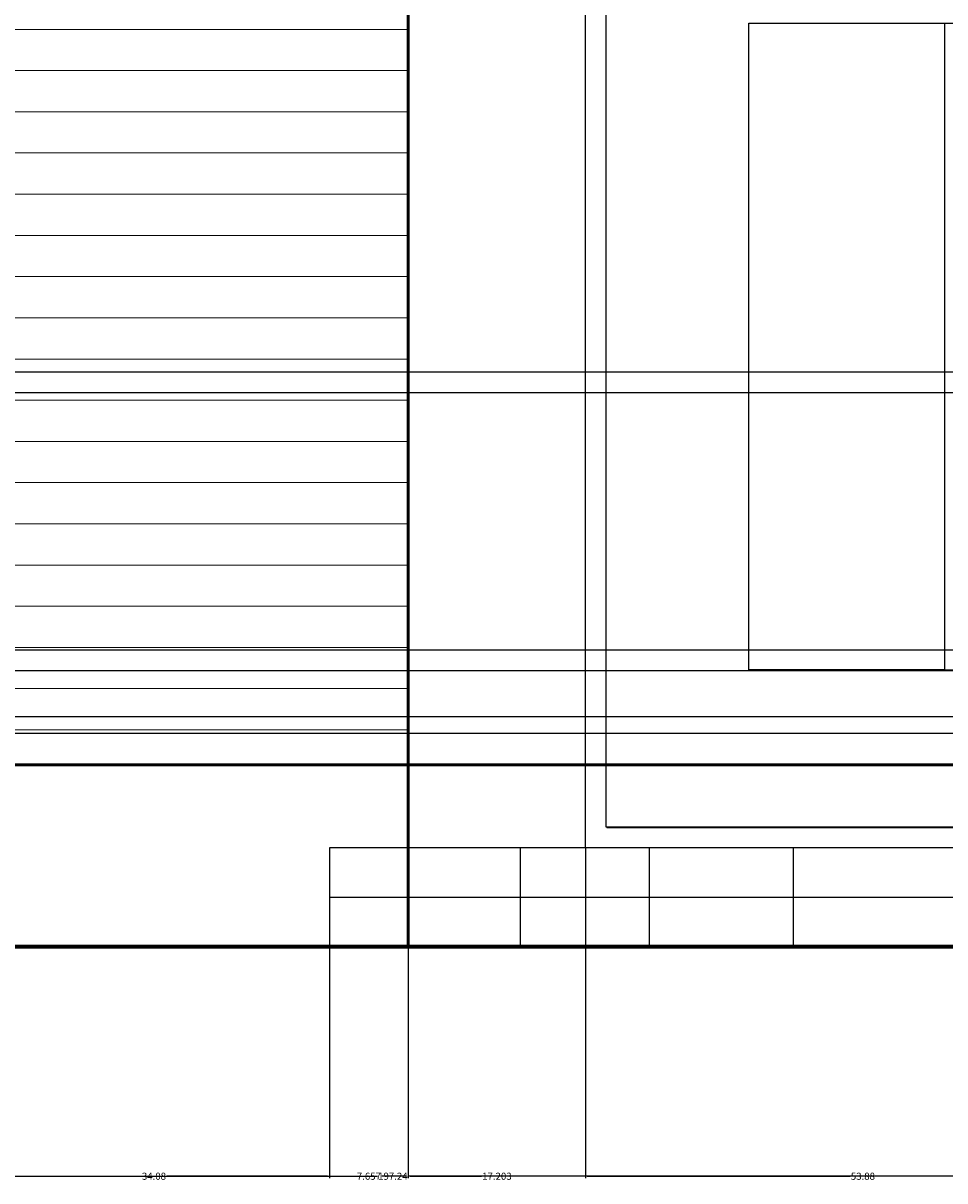
# Model space of a CAD drawing. Units: inches. Extents: x -139 to 346, y 72 to 413.
# Tile 11 of 18: x 175 to 265, y 72 to 185. Entities that reach past the tile are written whole.
import ezdxf

# ---------------------------------------------------------------- set-up
doc = ezdxf.new("R2010")
doc.units = ezdxf.units.IN
doc.header["$MEASUREMENT"] = 0
for name, color, linetype, lineweight in [('A-ANNO-DIMS', 2, 'Continuous', 18), ('A-DOOR', 3, 'Continuous', 25), ('A-FLOR-STRS', 2, 'Continuous', 25), ('A-WALL', 7, 'Continuous', 50), ('A-WALL-PATT', 8, 'Continuous', 13), ('C-TOPO', 7, 'Continuous', 70)]:
    doc.layers.add(name, color=color, linetype=linetype, lineweight=lineweight)
doc.styles.get("Standard").update_dxf_attribs({"font": 'arial.ttf'})
doc.dimstyles.get("Standard").update_dxf_attribs({"dimtxt": 0.6875, "dimasz": 0.18, "dimexe": 0.18, "dimexo": 0.0625, "dimgap": 0.09, "dimtad": 0, "dimtih": 1, "dimtoh": 1, "dimdec": 4, "dimzin": 0, "dimdsep": 46, "dimlunit": 4, "dimtxsty": 'Standard', "dimcen": 0.09, "dimadec": 0, "dimazin": 0, "dimtfac": 1, "dimtdec": 4, "dimtofl": 0, "dimtmove": 0, "dimatfit": 3, "dimfxl": 1, "dimtolj": 1, "dimtzin": 0, "dimarcsym": 0})

# ---------------------------------------------------------------- blocks, each defined once
blk = doc.blocks.new('*D7')
at = {"layer": 'A-ANNO-DIMS', "color": 0, "lineweight": -2, "transparency": 16777216}
for p, q in [((-47.27, 95.04), (-47.27, 117.45)), ((-47.09, 117.27), (129.79, 117.27)), ((309.71, 117.27), (132.82, 117.27)), ((309.89, 95.04), (309.89, 117.45))]:
    blk.add_line(p, q, dxfattribs=at)
at = {"layer": 'A-ANNO-DIMS', "color": 0, "transparency": 16777216}
for points in [[(-47.09, 117.3), (-47.09, 117.24), (-47.27, 117.27)], [(309.71, 117.3), (309.71, 117.24), (309.89, 117.27)]]:
    blk.add_solid(points, dxfattribs=at)
at = {"layer": 'Defpoints', "color": 0, "transparency": 16777216}
for p in [(309.89, 117.27), (-47.27, 94.97), (309.89, 94.97)]:
    blk.add_point(p, dxfattribs=at)
at = {"layer": 'A-ANNO-DIMS', "color": 0, "transparency": 16777216, "insert": (131.31, 117.27), "char_height": 0.688, "attachment_point": 5}
blk.add_mtext('\\A1;357.16', dxfattribs=at)
blk = doc.blocks.new('*D11')
at = {"layer": 'A-ANNO-DIMS', "color": 0, "lineweight": -2, "transparency": 16777216}
for p, q in [((112.65, 112.54), (112.65, 72.49)), ((309.89, 94.91), (309.89, 72.49)), ((112.83, 72.67), (209.79, 72.67)), ((309.71, 72.67), (212.75, 72.67))]:
    blk.add_line(p, q, dxfattribs=at)
at = {"layer": 'A-ANNO-DIMS', "color": 0, "transparency": 16777216}
for points in [[(112.83, 72.7), (112.83, 72.64), (112.65, 72.67)], [(309.71, 72.7), (309.71, 72.64), (309.89, 72.67)]]:
    blk.add_solid(points, dxfattribs=at)
at = {"layer": 'Defpoints', "color": 0, "transparency": 16777216}
for p in [(112.65, 112.6), (309.89, 94.97), (309.89, 72.67)]:
    blk.add_point(p, dxfattribs=at)
at = {"layer": 'A-ANNO-DIMS', "color": 0, "transparency": 16777216, "insert": (211.27, 72.67), "char_height": 0.688, "attachment_point": 5}
blk.add_mtext('\\A1;197.24', dxfattribs=at)
blk = doc.blocks.new('*D16')
at = {"layer": 'A-ANNO-DIMS', "color": 0, "lineweight": -2, "transparency": 16777216}
for p, q in [((125.31, 115.68), (344.39, 115.68)), ((344.21, 115.5), (344.21, 114.58)), ((344.21, 112.78), (344.21, 113.7)), ((112.71, 112.6), (344.39, 112.6))]:
    blk.add_line(p, q, dxfattribs=at)
at = {"layer": 'A-ANNO-DIMS', "color": 0, "transparency": 16777216}
for points in [[(344.18, 115.5), (344.24, 115.5), (344.21, 115.68)], [(344.18, 112.78), (344.24, 112.78), (344.21, 112.6)]]:
    blk.add_solid(points, dxfattribs=at)
at = {"layer": 'Defpoints', "color": 0, "transparency": 16777216}
for p in [(125.25, 115.68), (344.21, 115.68), (112.65, 112.6)]:
    blk.add_point(p, dxfattribs=at)
at = {"layer": 'A-ANNO-DIMS', "color": 0, "transparency": 16777216, "insert": (344.21, 114.14), "char_height": 0.688, "attachment_point": 5}
blk.add_mtext('\\A1;3.072', dxfattribs=at)
blk = doc.blocks.new('*D18')
at = {"layer": 'A-ANNO-DIMS', "color": 0, "lineweight": -2, "transparency": 16777216}
for p, q in [((171.03, 115.61), (171.03, 72.49)), ((205.11, 94.91), (205.11, 72.49)), ((171.21, 72.67), (186.82, 72.67)), ((204.93, 72.67), (189.32, 72.67))]:
    blk.add_line(p, q, dxfattribs=at)
at = {"layer": 'A-ANNO-DIMS', "color": 0, "transparency": 16777216}
for points in [[(171.21, 72.7), (171.21, 72.64), (171.03, 72.67)], [(204.93, 72.7), (204.93, 72.64), (205.11, 72.67)]]:
    blk.add_solid(points, dxfattribs=at)
at = {"layer": 'Defpoints', "color": 0, "transparency": 16777216}
for p in [(171.03, 115.68), (205.11, 94.97), (205.11, 72.67)]:
    blk.add_point(p, dxfattribs=at)
at = {"layer": 'A-ANNO-DIMS', "color": 0, "transparency": 16777216, "insert": (188.07, 72.67), "char_height": 0.688, "attachment_point": 5}
blk.add_mtext('\\A1;34.08', dxfattribs=at)
blk = doc.blocks.new('*D19')
at = {"layer": 'A-ANNO-DIMS', "color": 0, "lineweight": -2, "transparency": 16777216}
for p, q in [((205.11, 94.91), (205.11, 72.49)), ((212.77, 94.91), (212.77, 72.49)), ((205.29, 72.67), (207.69, 72.67)), ((212.59, 72.67), (210.19, 72.67))]:
    blk.add_line(p, q, dxfattribs=at)
at = {"layer": 'A-ANNO-DIMS', "color": 0, "transparency": 16777216}
for points in [[(205.29, 72.7), (205.29, 72.64), (205.11, 72.67)], [(212.59, 72.7), (212.59, 72.64), (212.77, 72.67)]]:
    blk.add_solid(points, dxfattribs=at)
at = {"layer": 'Defpoints', "color": 0, "transparency": 16777216}
for p in [(205.11, 94.97), (212.77, 94.97), (212.77, 72.67)]:
    blk.add_point(p, dxfattribs=at)
at = {"layer": 'A-ANNO-DIMS', "color": 0, "transparency": 16777216, "insert": (208.94, 72.67), "char_height": 0.688, "attachment_point": 5}
blk.add_mtext('\\A1;7.657', dxfattribs=at)
blk = doc.blocks.new('*D20')
at = {"layer": 'A-ANNO-DIMS', "color": 0, "lineweight": -2, "transparency": 16777216}
for p, q in [((229.97, 104.48), (229.97, 72.49)), ((212.77, 94.91), (212.77, 72.49)), ((212.95, 72.67), (219.89, 72.67)), ((229.79, 72.67), (222.86, 72.67))]:
    blk.add_line(p, q, dxfattribs=at)
at = {"layer": 'A-ANNO-DIMS', "color": 0, "transparency": 16777216}
for points in [[(212.95, 72.7), (212.95, 72.64), (212.77, 72.67)], [(229.79, 72.7), (229.79, 72.64), (229.97, 72.67)]]:
    blk.add_solid(points, dxfattribs=at)
at = {"layer": 'Defpoints', "color": 0, "transparency": 16777216}
for p in [(229.97, 104.54), (212.77, 94.97), (229.97, 72.67)]:
    blk.add_point(p, dxfattribs=at)
at = {"layer": 'A-ANNO-DIMS', "color": 0, "transparency": 16777216, "insert": (221.37, 72.67), "char_height": 0.688, "attachment_point": 5}
blk.add_mtext('\\A1;17.203', dxfattribs=at)
blk = doc.blocks.new('*D21')
at = {"layer": 'A-ANNO-DIMS', "color": 0, "lineweight": -2, "transparency": 16777216}
for p, q in [((229.97, 104.48), (229.97, 72.49)), ((283.85, 104.48), (283.85, 72.49)), ((230.15, 72.67), (255.66, 72.67)), ((283.67, 72.67), (258.16, 72.67))]:
    blk.add_line(p, q, dxfattribs=at)
at = {"layer": 'A-ANNO-DIMS', "color": 0, "transparency": 16777216}
for points in [[(230.15, 72.7), (230.15, 72.64), (229.97, 72.67)], [(283.67, 72.7), (283.67, 72.64), (283.85, 72.67)]]:
    blk.add_solid(points, dxfattribs=at)
at = {"layer": 'Defpoints', "color": 0, "transparency": 16777216}
for p in [(229.97, 104.54), (283.85, 104.54), (283.85, 72.67)]:
    blk.add_point(p, dxfattribs=at)
at = {"layer": 'A-ANNO-DIMS', "color": 0, "transparency": 16777216, "insert": (256.91, 72.67), "char_height": 0.688, "attachment_point": 5}
blk.add_mtext('\\A1;53.88', dxfattribs=at)
blk = doc.blocks.new('*D62')
at = {"layer": 'A-ANNO-DIMS', "color": 0, "lineweight": -2, "transparency": 16777216}
for p, q in [((55.33, 123.78), (344.39, 123.78)), ((344.21, 123.6), (344.21, 123.21)), ((57.33, 121.78), (344.39, 121.78)), ((344.21, 121.96), (344.21, 122.34))]:
    blk.add_line(p, q, dxfattribs=at)
at = {"layer": 'A-ANNO-DIMS', "color": 0, "transparency": 16777216}
for points in [[(344.18, 123.6), (344.24, 123.6), (344.21, 123.78)], [(344.18, 121.96), (344.24, 121.96), (344.21, 121.78)]]:
    blk.add_solid(points, dxfattribs=at)
at = {"layer": 'Defpoints', "color": 0, "transparency": 16777216}
for p in [(55.27, 123.78), (344.21, 123.78), (57.27, 121.78)]:
    blk.add_point(p, dxfattribs=at)
at = {"layer": 'A-ANNO-DIMS', "color": 0, "transparency": 16777216, "insert": (344.21, 122.78), "char_height": 0.688, "attachment_point": 5}
blk.add_mtext('\\A1;2', dxfattribs=at)
blk = doc.blocks.new('*D63')
at = {"layer": 'A-ANNO-DIMS', "color": 0, "lineweight": -2, "transparency": 16777216}
for p, q in [((55.33, 148.76), (344.39, 148.76)), ((344.21, 148.58), (344.21, 136.71)), ((344.21, 123.96), (344.21, 135.83)), ((55.33, 123.78), (344.39, 123.78))]:
    blk.add_line(p, q, dxfattribs=at)
at = {"layer": 'A-ANNO-DIMS', "color": 0, "transparency": 16777216}
for points in [[(344.18, 148.58), (344.24, 148.58), (344.21, 148.76)], [(344.18, 123.96), (344.24, 123.96), (344.21, 123.78)]]:
    blk.add_solid(points, dxfattribs=at)
at = {"layer": 'Defpoints', "color": 0, "transparency": 16777216}
for p in [(55.27, 148.76), (344.21, 148.76), (55.27, 123.78)]:
    blk.add_point(p, dxfattribs=at)
at = {"layer": 'A-ANNO-DIMS', "color": 0, "transparency": 16777216, "insert": (344.21, 136.27), "char_height": 0.688, "attachment_point": 5}
blk.add_mtext('\\A1;24.98', dxfattribs=at)
blk = doc.blocks.new('*D64')
at = {"layer": 'A-ANNO-DIMS', "color": 0, "lineweight": -2, "transparency": 16777216}
for p, q in [((55.33, 150.76), (344.39, 150.76)), ((344.21, 150.58), (344.21, 150.19)), ((55.33, 148.76), (344.39, 148.76)), ((344.21, 148.94), (344.21, 149.32))]:
    blk.add_line(p, q, dxfattribs=at)
at = {"layer": 'A-ANNO-DIMS', "color": 0, "transparency": 16777216}
for points in [[(344.18, 150.58), (344.24, 150.58), (344.21, 150.76)], [(344.18, 148.94), (344.24, 148.94), (344.21, 148.76)]]:
    blk.add_solid(points, dxfattribs=at)
at = {"layer": 'Defpoints', "color": 0, "transparency": 16777216}
for p in [(55.27, 150.76), (344.21, 150.76), (55.27, 148.76)]:
    blk.add_point(p, dxfattribs=at)
at = {"layer": 'A-ANNO-DIMS', "color": 0, "transparency": 16777216, "insert": (344.21, 149.76), "char_height": 0.688, "attachment_point": 5}
blk.add_mtext('\\A1;2', dxfattribs=at)
blk = doc.blocks.new('*D65')
at = {"layer": 'A-ANNO-DIMS', "color": 0, "lineweight": -2, "transparency": 16777216}
for p, q in [((55.33, 205.52), (344.39, 205.52)), ((344.21, 205.34), (344.21, 178.58)), ((344.21, 150.94), (344.21, 177.7)), ((55.33, 150.76), (344.39, 150.76))]:
    blk.add_line(p, q, dxfattribs=at)
at = {"layer": 'A-ANNO-DIMS', "color": 0, "transparency": 16777216}
for points in [[(344.18, 205.34), (344.24, 205.34), (344.21, 205.52)], [(344.18, 150.94), (344.24, 150.94), (344.21, 150.76)]]:
    blk.add_solid(points, dxfattribs=at)
at = {"layer": 'Defpoints', "color": 0, "transparency": 16777216}
for p in [(55.27, 205.52), (344.21, 205.52), (55.27, 150.76)]:
    blk.add_point(p, dxfattribs=at)
at = {"layer": 'A-ANNO-DIMS', "color": 0, "transparency": 16777216, "insert": (344.21, 178.14), "char_height": 0.688, "attachment_point": 5}
blk.add_mtext('\\A1;54.77', dxfattribs=at)
blk = doc.blocks.new('*D67')
at = {"layer": 'A-ANNO-DIMS', "color": 0, "lineweight": -2, "transparency": 16777216}
for p, q in [((57.33, 207.52), (344.39, 207.52)), ((344.21, 207.34), (344.21, 165.09)), ((344.21, 121.96), (344.21, 164.21)), ((57.33, 121.78), (344.39, 121.78))]:
    blk.add_line(p, q, dxfattribs=at)
at = {"layer": 'A-ANNO-DIMS', "color": 0, "transparency": 16777216}
for points in [[(344.18, 207.34), (344.24, 207.34), (344.21, 207.52)], [(344.18, 121.96), (344.24, 121.96), (344.21, 121.78)]]:
    blk.add_solid(points, dxfattribs=at)
at = {"layer": 'Defpoints', "color": 0, "transparency": 16777216}
for p in [(57.27, 207.52), (344.21, 207.52), (57.27, 121.78)]:
    blk.add_point(p, dxfattribs=at)
at = {"layer": 'A-ANNO-DIMS', "color": 0, "transparency": 16777216, "insert": (344.21, 164.65), "char_height": 0.688, "attachment_point": 5}
blk.add_mtext('\\A1;85.75', dxfattribs=at)
blk = doc.blocks.new('*D83')
at = {"layer": 'A-ANNO-DIMS', "color": 0, "lineweight": -2, "transparency": 16777216}
for p, q in [((245.9, 121.84), (344.39, 121.84)), ((344.21, 121.66), (344.21, 114.63)), ((344.21, 106.72), (344.21, 113.75)), ((232.03, 106.54), (344.39, 106.54))]:
    blk.add_line(p, q, dxfattribs=at)
at = {"layer": 'A-ANNO-DIMS', "color": 0, "transparency": 16777216}
for points in [[(344.18, 121.66), (344.24, 121.66), (344.21, 121.84)], [(344.18, 106.72), (344.24, 106.72), (344.21, 106.54)]]:
    blk.add_solid(points, dxfattribs=at)
at = {"layer": 'Defpoints', "color": 0, "transparency": 16777216}
for p in [(245.84, 121.84), (344.21, 121.84), (231.97, 106.54)]:
    blk.add_point(p, dxfattribs=at)
at = {"layer": 'A-ANNO-DIMS', "color": 0, "transparency": 16777216, "insert": (344.21, 114.19), "char_height": 0.688, "attachment_point": 5}
blk.add_mtext('\\A1;15.3', dxfattribs=at)
blk = doc.blocks.new('*D84')
at = {"layer": 'A-ANNO-DIMS', "color": 0, "lineweight": -2, "transparency": 16777216}
for p, q in [((245.9, 184.61), (344.39, 184.61)), ((344.21, 184.43), (344.21, 153.67)), ((344.21, 122.02), (344.21, 152.78)), ((245.9, 121.84), (344.39, 121.84))]:
    blk.add_line(p, q, dxfattribs=at)
at = {"layer": 'A-ANNO-DIMS', "color": 0, "transparency": 16777216}
for points in [[(344.18, 184.43), (344.24, 184.43), (344.21, 184.61)], [(344.18, 122.02), (344.24, 122.02), (344.21, 121.84)]]:
    blk.add_solid(points, dxfattribs=at)
at = {"layer": 'Defpoints', "color": 0, "transparency": 16777216}
for p in [(245.84, 184.61), (344.21, 184.61), (245.84, 121.84)]:
    blk.add_point(p, dxfattribs=at)
at = {"layer": 'A-ANNO-DIMS', "color": 0, "transparency": 16777216, "insert": (344.21, 153.22), "char_height": 0.688, "attachment_point": 5}
blk.add_mtext('\\A1;62.76', dxfattribs=at)

msp = doc.modelspace()

# ---------------------------------------------------------------- hatches: boundary and pattern name
at = {"layer": 'A-WALL-PATT'}
h = msp.add_hatch(dxfattribs=at)
h.set_pattern_fill('ANSI31', color=256, scale=32, angle=135)
h.paths.add_polyline_path([(98.6724, 360.5443), (-34.7346, 360.5443), (-34.7346, 353.0644), (-34.7346, 305.9205), (5.6729, 305.9205), (5.6729, 338.3217), (62.4258, 338.3217), (62.4258, 305.9205), (98.6724, 305.9205)])
h.paths.add_polyline_path([(212.769, 231.0607), (175.072, 231.0607), (175.072, 218.0635), (171.0337, 218.0635), (171.0337, 115.6761), (125.2464, 115.6761), (125.2464, 218.0635), (123.4318, 218.0635), (120.5054, 218.0635), (120.5054, 231.0607), (112.6506, 231.0607), (112.6506, 112.6042), (212.769, 112.6042)])

# ---------------------------------------------------------------- linework, layer by layer
at = {"layer": 'A-DOOR'}
for points in [[(229.972, 205.5243), (283.8497, 205.5243), (283.8497, 104.5429), (229.972, 104.5429)], [(231.972, 203.5243), (281.8497, 203.5243), (281.8497, 106.5429), (231.972, 106.5429)], [(245.8399, 184.6055), (264.8219, 184.6055), (264.8219, 121.8428), (245.8399, 121.8428)]]:
    msp.add_lwpolyline(points, close=True, dxfattribs=at)
at = {"layer": 'A-FLOR-STRS'}
for p, q in [((229.972, 104.5429), (205.1121, 104.5429)), ((205.1121, 104.5429), (205.1121, 94.9748)), ((223.6353, 104.5429), (223.6353, 94.9748)), ((236.1693, 104.5429), (236.1693, 94.9748)), ((250.1238, 104.5429), (250.1238, 94.9748)), ((205.1121, 99.7588), (292.1669, 99.7588))]:
    msp.add_line(p, q, dxfattribs=at)
at = {"layer": 'A-WALL'}
for p, q in [((212.769, 231.0607), (212.769, 94.9748)), ((112.6506, 112.6042), (297.5013, 112.6042))]:
    msp.add_line(p, q, dxfattribs=at)
at = {"layer": 'C-TOPO'}
msp.add_line((51.0187, 94.9748), (321.9055, 94.9748), dxfattribs=at)

# ---------------------------------------------------------------- dimensions: what is measured, and where the dimension line sits
at = {"layer": 'A-ANNO-DIMS'}
for base, p1, p2, override, picture, middle in [((344.2055, 207.5243), (57.2654, 121.7753), (57.2654, 207.5243), {"dimdec": 2, "dimlfac": 1, "dimrnd": 0, "dimzin": 0, "dimdsep": 46, "dimlunit": 2}, '*D67', (344.2055, 164.6498)), ((344.2055, 205.5243), (55.2654, 150.7576), (55.2654, 205.5243), {"dimdec": 2, "dimlfac": 1, "dimrnd": 0, "dimzin": 0, "dimdsep": 46, "dimlunit": 2}, '*D65', (344.2055, 178.141)), ((344.2055, 184.6055), (245.8399, 121.8428), (245.8399, 184.6055), {"dimdec": 2, "dimlfac": 1, "dimrnd": 0, "dimzin": 0, "dimdsep": 46, "dimlunit": 2}, '*D84', (344.2055, 153.2242)), ((344.2055, 150.7576), (55.2654, 148.7576), (55.2654, 150.7576), {"dimdec": 0, "dimlfac": 1, "dimrnd": 0, "dimzin": 0, "dimdsep": 46, "dimlunit": 2}, '*D64', (344.2055, 149.7576)), ((344.2055, 148.7576), (55.2654, 123.7753), (55.2654, 148.7576), {"dimdec": 2, "dimlfac": 1, "dimrnd": 0, "dimzin": 0, "dimdsep": 46, "dimlunit": 2}, '*D63', (344.2055, 136.2665)), ((344.2055, 123.7753), (57.2654, 121.7753), (55.2654, 123.7753), {"dimdec": 0, "dimlfac": 1, "dimrnd": 0, "dimzin": 0, "dimdsep": 46, "dimlunit": 2}, '*D62', (344.2055, 122.7753)), ((344.2055, 121.8428), (231.972, 106.5429), (245.8399, 121.8428), {"dimdec": 1, "dimlfac": 1, "dimrnd": 0, "dimzin": 0, "dimdsep": 46, "dimlunit": 2}, '*D83', (344.2055, 114.1929)), ((344.2055, 115.6761), (112.6506, 112.6042), (125.2464, 115.6761), {"dimdec": 3, "dimlfac": 1, "dimrnd": 0, "dimzin": 0, "dimdsep": 46, "dimlunit": 2}, '*D16', (344.2055, 114.1402))]:
    dim = msp.add_linear_dim(base=base, p1=p1, p2=p2, angle=90, dimstyle='Standard', override=override, dxfattribs=at)
    dim.commit()
    dim.dimension.update_dxf_attribs({"geometry": picture, "text_midpoint": middle})
for base, p1, p2, override, picture, middle in [((309.8894, 117.2748), (-47.2734, 94.9748), (309.8894, 94.9748), {"dimdec": 2, "dimlfac": 1, "dimrnd": 0, "dimzin": 0, "dimdsep": 46, "dimlunit": 2}, '*D7', (131.308, 117.2748)), ((205.1121, 72.6748), (171.0337, 115.6761), (205.1121, 94.9748), {"dimdec": 2, "dimlfac": 1, "dimrnd": 0, "dimzin": 0, "dimdsep": 46, "dimlunit": 2}, '*D18', (188.0729, 72.6748)), ((309.8894, 72.6748), (112.6506, 112.6042), (309.8894, 94.9748), {"dimdec": 2, "dimlfac": 1, "dimrnd": 0, "dimzin": 0, "dimdsep": 46, "dimlunit": 2}, '*D11', (211.27, 72.6748)), ((229.972, 72.6748), (212.769, 94.9748), (229.972, 104.5429), {"dimdec": 3, "dimlfac": 1, "dimrnd": 0, "dimzin": 0, "dimdsep": 46, "dimlunit": 2}, '*D20', (221.3705, 72.6748)), ((283.8497, 72.6748), (229.972, 104.5429), (283.8497, 104.5429), {"dimdec": 2, "dimlfac": 1, "dimrnd": 0, "dimzin": 0, "dimdsep": 46, "dimlunit": 2}, '*D21', (256.9109, 72.6748)), ((212.769, 72.6748), (205.1121, 94.9748), (212.769, 94.9748), {"dimdec": 3, "dimlfac": 1, "dimrnd": 0, "dimzin": 0, "dimdsep": 46, "dimlunit": 2}, '*D19', (208.9406, 72.6748))]:
    dim = msp.add_linear_dim(base=base, p1=p1, p2=p2, dimstyle='Standard', override=override, dxfattribs=at)
    dim.commit()
    dim.dimension.update_dxf_attribs({"geometry": picture, "text_midpoint": middle})

doc.saveas('drawing.dxf')
